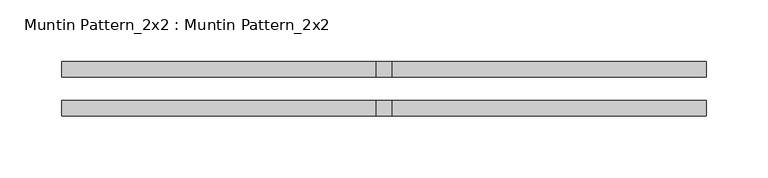
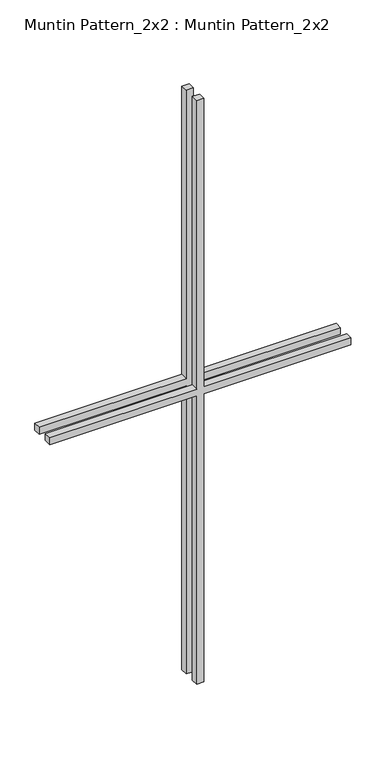
"""IFC4 building model written with IfcOpenShell, lengths in millimetres: proxy geometry, Muntin Pattern_2x2 : Muntin Pattern_2x2."""

from ifc_helpers import new_model, si_unit, frame, origin, place, context, project, spatial, polyline, outline, extrude, source, transform, mapped, element, save


def muntin_pattern_2x2_muntin_pattern_2x2_cf37b409(model_context):
    return source(origin(), model_context, "Body", "SweptSolid", [
        extrude(outline(polyline([(542.925, -6.35), (542.925, -261.9375), (530.225, -261.9375), (530.225, -6.35), (0.0, -6.35), (0.0, 6.35), (530.225, 6.35), (530.225, 261.9375), (542.925, 261.9375), (542.925, 6.35), (1073.15, 6.35), (1073.15, -6.35), (542.925, -6.35)])), frame((0.0, 9.525, 0.0), z_axis=(0.0, 1.0, 0.0), x_axis=(0.0, 0.0, 1.0)), (0.0, 0.0, 1.0), 12.7),
        extrude(outline(polyline([(542.925, -6.35), (542.925, -261.9375), (530.225, -261.9375), (530.225, -6.35), (0.0, -6.35), (0.0, 6.35), (530.225, 6.35), (530.225, 261.9375), (542.925, 261.9375), (542.925, 6.35), (1073.15, 6.35), (1073.15, -6.35), (542.925, -6.35)])), frame((0.0, -22.225, 0.0), z_axis=(0.0, 1.0, 0.0), x_axis=(0.0, 0.0, 1.0)), (0.0, 0.0, 1.0), 12.7),
    ])


if __name__ == "__main__":
    model = new_model("IFC4")
    model_context = context("Model", 3, world=origin())
    ifc_project = project(units=[si_unit("LENGTHUNIT", "METRE", prefix="MILLI")], contexts=[model_context])
    site = spatial("IfcSite", under=ifc_project)
    building = spatial("IfcBuilding", under=site)
    placement = place(None, origin())
    muntin_pattern_2x2_muntin_pattern_2x2_shape = muntin_pattern_2x2_muntin_pattern_2x2_cf37b409(model_context)
    element("IfcBuildingElementProxy", 1, Name="Muntin Pattern_2x2 : Muntin Pattern_2x2", ObjectType="Muntin Pattern_2x2 : Muntin Pattern_2x2", at=placement, inside=building, context=model_context, shape_type="MappedRepresentation", body=[
        mapped(muntin_pattern_2x2_muntin_pattern_2x2_shape, transform((0.0, 0.0, 0.0), x_axis=(1.0, 0.0, 0.0), y_axis=(0.0, 1.0, 0.0), z_axis=(0.0, 0.0, 1.0))),
    ])
    save(model, "model.ifc")

# Revit data of these elements
# Type "Muntin Pattern_2x2 : Muntin Pattern_2x2"
#   Width [instance default] = 4' - 0"
#   Thickness = 0' - 0 1/2"
#   Height [instance default] = 4' - 0"
#   Distance = 0' - 0 3/4"
#   Interior Material [instance default] = none
#   Exterior Material [instance default] = none
#   Default Elevation = 0
# Element 1 (IfcBuildingElementProxy, "Muntin Pattern_2x2 : Muntin Pattern_2x2")
#   Width = 1' - 8 5/8"
#   Height = 3' - 6 1/4"
#   Interior Material = Wood - Stained
#   Exterior Material = Clad - White
#   Materials on its faces: "Clad - White", "Wood - Stained"
# Materials
#   "Clad - White": class "Wood", colour RGB 242 242 238, transparency 0, Cost = 0
#   "Wood - Stained": class "Wood", colour RGB 224 178 126, transparency 0, Cost = 0
